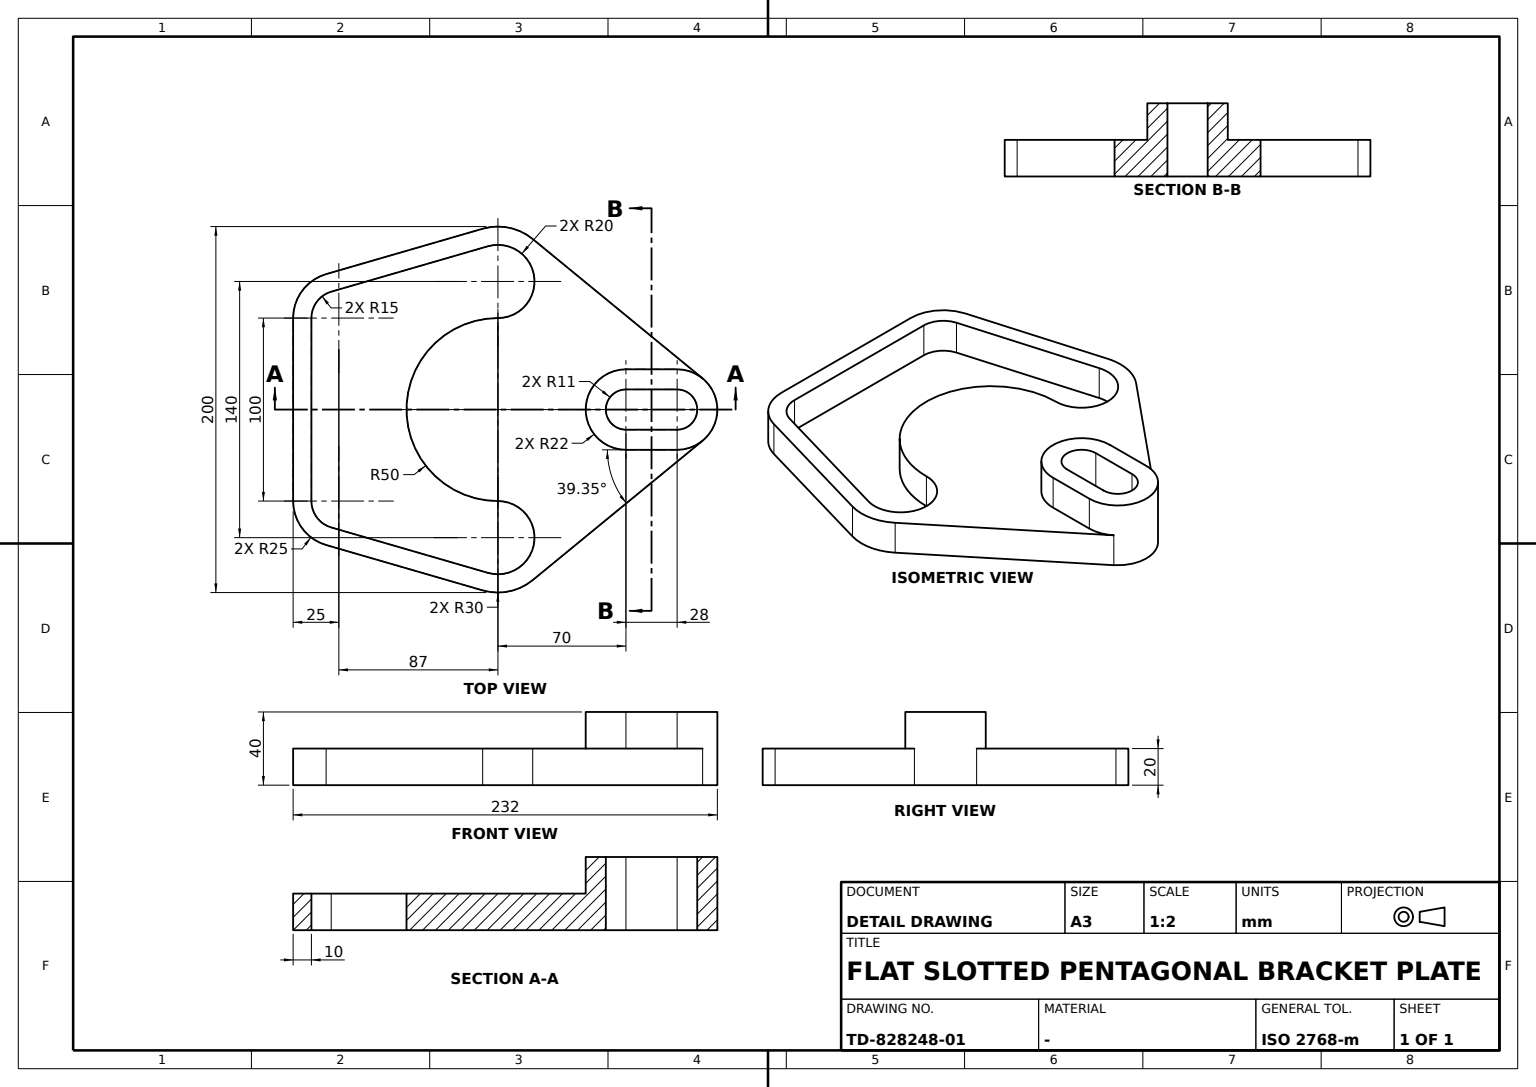
CATIA V5 part; units mm, degrees
sketch "Sketch1" plane through (0, 0, 0) normal (0, 0, 1) x (1, 0, 0)
  arc A0 (-50, 0) -> (50, 0) centre (0, 0) ccw
  line L0 (0, 174.8369) -> (0, -177.8743) construction
  point P0 (0, 174.8369)
  line L1 (50, -102) -> (-50, -102)
  point P1 (50, -102)
  line L2 (64.4075, -91.1741) -> (89.21, -5.5655)
  line L3 (-64.4075, -91.1741) -> (-89.21, -5.5655)
  arc A1 (50, -102) -> (64.4075, -91.1741) centre (50, -87) ccw
  point P2 (50, -87)
  arc A2 (89.21, -5.5655) -> (50, 0) centre (70, 0) ccw
  point P3 (70, 0)
  arc A3 (-50, 0) -> (-89.21, -5.5655) centre (-70, 0) ccw
  point P4 (-70, 0)
  arc A4 (-64.4075, -91.1741) -> (-50, -102) centre (-50, -87) ccw
  point P5 (-50, -87)
  arc A5 (-93.1998, 19.0203) -> (-98.815, -8.3483) centre (-70, 0) ccw
  line L4 (-74.0125, -93.9569) -> (-98.815, -8.3483)
  arc A6 (-74.0125, -93.9569) -> (-50, -112) centre (-50, -87) ccw
  line L5 (50, -112) -> (-50, -112)
  arc A7 (50, -112) -> (74.0125, -93.9569) centre (50, -87) ccw
  line L6 (74.0125, -93.9569) -> (98.815, -8.3483)
  arc A8 (98.815, -8.3483) -> (93.1998, 19.0203) centre (70, 0) ccw
  line L7 (0, 98) -> (0, 70) construction
  point P6 (0, 98)
  point P7 (0, 70)
  arc A9 (-17.0132, 111.9482) -> (17.0132, 111.9482) centre (0, 98) cw
  line L8 (17.0132, 111.9482) -> (93.1998, 19.0203)
  point P8 (93.1998, 19.0203)
  point P9 (17.0132, 111.9482)
  point P10 (-93.1998, 19.0203)
  point P11 (-17.0132, 111.9482)
  line L9 (-17.0132, 111.9482) -> (-93.1998, 19.0203)
  dimension "radius A0" = 50
  dimension "radius A1" = 15
  dimension "radius A2" = 20
  dimension "radius A3" = 20
  dimension "distance P3 L0" = 70
  dimension "distance L0 P4" = 70
  dimension "radius A4" = 15
  dimension "distance P2 x axis" = 87
  dimension "distance P2 P5" = 100
  dimension "distance L0 P2" = 50
  dimension "radius A7" = 25
  dimension "length L5" = 100
  dimension "radius A6" = 25
  dimension "distance x axis L5" = 112
  dimension "distance L3 L4" = 10
  dimension "distance L6 L2" = 10
  dimension "distance A1 A7" = 10
  dimension "distance A4 A6" = 10
  dimension "radius A9" = 22
  dimension "distance P6 P7" = 28
  dimension "distance P7 x axis" = 70
  dimension "radius A8" = 30
  dimension "radius A5" = 30
  dimension "angle L8 L0" = 39.346
  dimension "distance A8 A2" = 10
  dimension "distance A3 A5" = 10
  constraint coincidence P0 y-axis
  constraint coincidence P3 x-axis
  constraint coincidence P4 x-axis
  constraint coincidence P6 L0
  constraint vertical L0 y-axis
  constraint vertical L7 y-axis
  constraint horizontal L1 x-axis
  constraint tangency A1 L2
  constraint tangency A1 L1
  constraint tangency L2 A2
  constraint tangency L3 A3
  constraint tangency A4 L1
  constraint tangency A4 L3
  constraint tangency L8 A8
  constraint tangency L8 A9
  constraint symmetry P8 P10 L7
  constraint symmetry P9 P11 L7
  constraint symmetry L8 L9 L7
extrude "Pad1" add sketch "Sketch1" against normal blind 20
sketch "Sketch2" plane through (0, 0, 0) normal (0, 0, 1) x (1, 0, 0)
  line L0 (0, 70) -> (0, 98) construction
  point P0 (0, 70)
  line L1 (-22, 70) -> (-22, 98)
  line L2 (22, 98) -> (22, 70)
  arc A0 (-22, 98) -> (22, 98) centre (0, 98) cw
  arc A1 (22, 70) -> (-22, 70) centre (0, 70) cw
  arc A2 (17.0132, 111.9482) -> (-17.0132, 111.9482) centre (0, 98) ccw construction
  line L3 (0, 98) -> (0, 70) construction
  line L4 (11, 98) -> (11, 70)
  line L5 (-11, 70) -> (-11, 98)
  arc A3 (11, 70) -> (-11, 70) centre (0, 70) cw
  arc A4 (-11, 98) -> (11, 98) centre (0, 98) cw
  dimension "radius A0" = 22
  dimension "length L0" = 28
  dimension "radius A4" = 11
  dimension "radius A1" = 22
  dimension "radius A3" = 11
  constraint coincidence P0 y-axis
  constraint vertical L0 y-axis
  constraint vertical L3 y-axis
  constraint tangency A0 L1
  constraint tangency A1 L1
  constraint tangency A0 L2
  constraint tangency A1 L2
  constraint tangency A3 L4
  constraint tangency A4 L4
  constraint tangency A3 L5
  constraint tangency A4 L5
  constraint concentricity A0 A2
extrude "Pad2" add sketch "Sketch2" along normal blind 20
sketch "Sketch3" plane through (0, 0, 0) normal (0, 0, 1) x (1, 0, 0)
  line L0 (11, 70) -> (11, 98)
  point P0 (11, 70)
  line L1 (-11, 98) -> (-11, 70)
  point P1 (-11, 70)
  arc A0 (11, 98) -> (-11, 98) centre (0, 98) ccw
  point P2 (0, 98)
  arc A1 (-11, 70) -> (11, 70) centre (0, 70) ccw
  point P3 (0, 70)
  point P4 (-11, 70)
  point P5 (11, 70)
  constraint coincidence P2 y-axis
  constraint coincidence A1 P1
  constraint coincidence P3 y-axis
  constraint coincidence L0 P5
  constraint coincidence L1 P4
  constraint coincidence P0 P5
  constraint coincidence P1 P4
  constraint tangency A0 L0
  constraint tangency A1 L0
extrude "Pocket1" cut sketch "Sketch3" against normal blind 20
